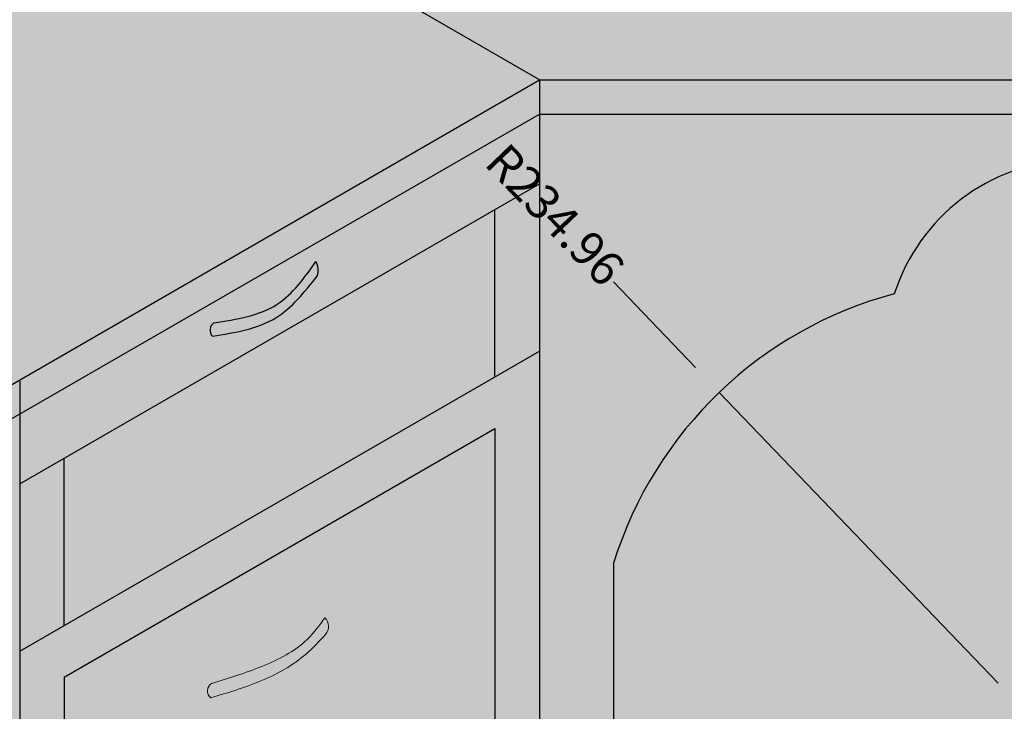
# Model space of a CAD drawing. Units: millimetres. Extents: x 78378 to 86415, y 148682 to 152721.
# Tile 8 of 18: x 79783 to 80358, y 150092 to 150495. Entities that reach past the tile are written whole.
import ezdxf

# ---------------------------------------------------------------- set-up
doc = ezdxf.new("R2010")
doc.units = ezdxf.units.MM
for name, color, linetype, lineweight in [('A-ANNO-DIMS', 2, 'Continuous', 18), ('A-FURN', 4, 'Continuous', 25), ('A-FURN-HRDW', 8, 'Continuous', 18), ('A-FURN-PATT', 32, 'Continuous', 13)]:
    doc.layers.add(name, color=color, linetype=linetype, lineweight=lineweight)
doc.styles.get("Standard").update_dxf_attribs({"font": 'arial.ttf'})
doc.dimstyles.new('ISO-25', dxfattribs={"dimtxt": 20, "dimasz": 20, "dimexe": 1.25, "dimexo": 0.625, "dimtad": 0, "dimdec": 1, "dimtxsty": 'Standard', "dimcen": 2.5, "dimadec": 0, "dimazin": 0, "dimtfac": 1, "dimtdec": 1, "dimtmove": 0, "dimatfit": 3, "dimfxl": 1, "dimarcsym": 0})

# ---------------------------------------------------------------- blocks, each defined once
blk = doc.blocks.new('HANDLE-DRAWER')
for centre, radius, start, end in [((63.38622997708444, 41.62154367045149), 7.231969022595942, 319.3237562697811, 44.69265733271547), ((5.163435732683865, 4.025219173752702), 5.172557027146686, 122.0794663418697, 231.0916038547452)]:
    blk.add_arc(centre, radius, start, end)
for points, knots in [([(2.416316796850878, 8.407990414794767), (12.22361058796001, 11.4080339887645), (31.81170594566225, 17.4000171857454), (55.97206586949582, 29.46692429189343), (65.30177131113433, 42.2784439569471), (68.52736162004294, 46.70781355843064)], [0, 0, 0, 0, 30.92804236988506, 61.77253950703249, 78.07166049105084, 78.07166049105084, 78.07166049105084, 78.07166049105084]), ([(1.914671141596045, 0.0001881390053313), (11.78696018195832, 2.942018891461464), (31.50487046795086, 8.817733694416148), (54.70585002572761, 21.54120260495396), (65.2835446695137, 33.01612223177024), (68.87098889380286, 36.90786192796077)], [0, 0, 0, 0, 30.92804236988506, 61.77253950704738, 77.60214595393334, 77.60214595393334, 77.60214595393334, 77.60214595393334])]:
    blk.add_open_spline(points, degree=3, knots=knots)
blk = doc.blocks.new('*D32')
at = {"layer": 'A-ANNO-DIMS', "color": 0, "lineweight": -2, "transparency": 16777216}
for p, q in [((80086.404202, 150459.382643), (80086.404202, 148693.757643)), ((80692.621985, 150459.382643), (80692.621985, 148693.757643)), ((80106.404202, 148695.007643), (80355.19095843862, 148695.007643)), ((80672.621985, 148695.007643), (80423.8352285614, 148695.007643))]:
    blk.add_line(p, q, dxfattribs=at)
at = {"layer": 'A-ANNO-DIMS', "color": 0, "transparency": 16777216}
for points in [[(80106.404202, 148698.3409763333), (80106.404202, 148691.6743096666), (80086.404202, 148695.007643)], [(80672.621985, 148698.3409763333), (80672.621985, 148691.6743096666), (80692.621985, 148695.007643)]]:
    blk.add_solid(points, dxfattribs=at)
at = {"layer": 'Defpoints', "color": 0, "transparency": 16777216}
for p in [(80086.404202, 150460.007643), (80692.621985, 150460.007643), (80692.621985, 148695.007643)]:
    blk.add_point(p, dxfattribs=at)
at = {"layer": 'A-ANNO-DIMS', "color": 0, "transparency": 16777216, "insert": (80389.5130935, 148695.007643), "char_height": 20, "attachment_point": 5}
blk.add_mtext('606.2', dxfattribs=at)
blk = doc.blocks.new('*D63')
at = {"layer": 'A-ANNO-DIMS', "color": 0, "lineweight": -2, "transparency": 16777216}
for p, q in [((80129.57071185744, 150342.1032015505), (80177.51998013844, 150292.103098691)), ((80353.993525, 150108.081617), (80191.36297800002, 150277.668023))]:
    blk.add_line(p, q, dxfattribs=at)
at = {"layer": 'A-ANNO-DIMS', "color": 0, "transparency": 16777216}
blk.add_solid([(80179.92582608695, 150294.4102650013), (80175.11413418995, 150289.7959323807), (80191.36297800002, 150277.668023)], dxfattribs=at)
at = {"layer": 'Defpoints', "color": 0, "transparency": 16777216}
for p in [(80191.36297800002, 150277.668023), (80353.993525, 150108.081617)]:
    blk.add_point(p, dxfattribs=at)
at = {"layer": 'A-ANNO-DIMS', "color": 0, "transparency": 16777216, "insert": (80093.78465023855, 150379.4198661427), "char_height": 20, "attachment_point": 5, "rotation": 313.8005333959761}
blk.add_mtext('R234.96', dxfattribs=at)

msp = doc.modelspace()

# ---------------------------------------------------------------- hatches: boundary and pattern name
at = {"layer": 'A-FURN-PATT'}
h = msp.add_hatch(color=256, dxfattribs=at)
h.dxf.hatch_style = 1
h.paths.add_polyline_path([(78839.32762104142, 151040.0076434961), (78579.5199999061, 151190.0076434961), (78579.51999990609, 150470.0076434961), (78839.3276210414, 150320.0076434962)])
h.paths.add_polyline_path([(79073.15448006323, 150899.6468812434, 0.2777796948118413), (79002.26445210895, 150996.320534414, 0.7910839311940991), (78917.95668085644, 150978.871860828, 0.1804483162531181), (78856.64812911711, 150853.0137915998), (78856.6481291171, 150350.6972986685), (79073.15448006321, 150484.3179883237)])
h.paths.add_polyline_path([(79073.15448006324, 151175.0076434962), (78856.64812911711, 151050.0076434961), (78856.64812911711, 150853.0137915998, -0.1804483162531142), (78917.95668085644, 150978.871860828, -0.7910839311941295), (79002.26445210895, 150996.320534414, -0.2777796948118357), (79073.15448006323, 150899.6468812434)])
h.paths.add_polyline_path([(79341.6223552364, 151350.0076434962), (79099.13524217675, 151490.0076434961), (78596.84050798177, 151200.0076434961), (78839.32762104142, 151060.0076434961)])
h.paths.add_polyline_path([(79904.53886769625, 151675.0076434962), (79662.05175463663, 151815.0076434961), (79099.13524217677, 151490.0076434961), (79341.62235523641, 151350.0076434962)])
h.paths.add_polyline_path([(80389.51309381555, 151955.0076434962), (80389.51309381555, 152235.0076434961), (79662.05175463663, 151815.0076434961), (79904.53886769625, 151675.0076434962)])
h.paths.add_polyline_path([(80389.51309381556, 151955.0076434962), (80164.3464888316, 151825.0076434962), (80164.3464888316, 151105.0076434962), (80614.67969879952, 151105.0076434962), (80614.6796987995, 151825.0076434962)])
edge = h.paths.add_edge_path(flags=16)
edge.add_spline(control_points=[(80216.30801305865, 151728.2510436129), (80227.18536059232, 151732.9809964381), (80256.33007611947, 151745.6544105326), (80298.40995723462, 151761.9595198717), (80340.25974320961, 151805.8549546823), (80391.07708467716, 151782.0404209196), (80454.03959007034, 151805.7580622626), (80496.50068603146, 151742.4094823368), (80543.82179764508, 151733.4042954735), (80562.71817457242, 151729.808323201)], knot_values=[0, 0, 0, 0, 35.54374676083332, 95.23575346876503, 136.367675126486, 200.9329819670103, 236.7264108107793, 322.8899349763893, 380.1702736670829, 380.1702736670829, 380.1702736670829, 380.1702736670829], degree=3, periodic=0)
edge.add_line((80562.71817457242, 151729.808323201), (80562.71817457245, 151165.0076434962))
edge.add_line((80562.71817457245, 151165.0076434962), (80216.30801305866, 151165.0076434962))
edge.add_line((80216.30801305866, 151165.0076434962), (80216.30801305865, 151728.2510436129))
h.paths.add_polyline_path([(80632.00020687516, 152095.0076434962), (80389.51309381555, 152235.0076434961), (80389.51309381555, 151955.0076434962), (80614.6796987995, 151825.0076434962), (80632.0002068752, 151815.0076434962)])
h.paths.add_polyline_path([(80867.77935513339, 151958.88048878), (80632.00020687516, 152095.0076434962), (80632.0002068752, 151815.0076434962), (80632.0002068752, 151510.0076434961), (80867.77935513335, 151373.88048878)])
h.paths.add_polyline_path([(80147.02598075592, 151495.8202891389, 0.1891897896548484), (80063.56711348135, 151597.7244306894, 0.7882613551016187), (79979.26906997921, 151580.5832085911, 0.1607261321771384), (79904.53886769625, 151413.5769349066), (79904.53886769625, 150955.0076434962), (80147.0259807559, 151095.0076434962)])
h.paths.add_polyline_path([(80147.02598075592, 151815.0076434961), (79904.53886769625, 151675.0076434962), (79904.53886769625, 151413.5769349066, -0.1607261321771371), (79979.26906997921, 151580.5832085911, -0.7882613551017736), (80063.56711348135, 151597.7244306894, -0.189189789654803), (80147.02598075592, 151495.820289139)])
h.paths.add_polyline_path([(79887.21835962054, 151645.0076434962), (79640.40111954202, 151502.5076434962), (79640.40111954202, 151262.3324568555, -0.160726132177166), (79715.13132182499, 151429.33873054, -0.7882613551016538), (79799.42936532712, 151446.4799526383, -0.2129057797217132), (79887.21835962054, 151328.7246881029)])
h.paths.add_polyline_path([(79799.42936532712, 151446.4799526383, 0.7882613551016341), (79715.13132182499, 151429.33873054, 0.1607261321772164), (79640.40111954202, 151262.3324568554), (79640.401119542, 150822.5076434962), (79887.21835962054, 150965.0076434962), (79887.21835962054, 151328.7246881029, 0.2129057797217146)])
h.paths.add_polyline_path([(79605.76010339064, 151482.5076434962), (79358.94286331208, 151340.0076434962), (79358.94286331208, 151100.0700856759, -0.1607261321769527), (79433.67306559504, 151267.0763593602, -0.7882613551016573), (79517.97110909715, 151284.2175814584, -0.2129057797218584), (79605.76010339064, 151166.4623169229)])
h.paths.add_polyline_path([(79605.76010339064, 151166.4623169229, 0.2129057797218619), (79517.97110909715, 151284.2175814584, 0.7882613551016192), (79433.67306559504, 151267.0763593602, 0.160726132177026), (79358.94286331208, 151100.0700856758), (79358.9428633121, 150742.9831021798), (79419.08774136574, 150694.7323050308), (79605.76010339062, 150802.5076434962)])
edge = h.paths.add_edge_path(flags=0)
edge.add_spline(control_points=[(81152.43559504113, 151098.7675637242), (81105.72083218757, 151145.9466131586), (81038.6136018851, 151213.7208057789), (80882.38658818699, 151214.1937625951), (80797.44342369089, 151311.2996726886), (80711.86856819791, 151340.3754369685), (80681.7690729932, 151350.6023409169)], knot_values=[0, 0, 0, 0, 188.2334409997391, 270.4032751997918, 445.4517920122014, 540.4285882874335, 540.4285882874335, 540.4285882874335, 540.4285882874335], degree=3, periodic=0)
edge.add_line((80683.45384528628, 151350.0268865391), (80683.45384528628, 151104.8791667058))
edge.add_line((80683.45384528628, 151104.8791667058), (81152.43559504113, 150851.3990036113))
edge.add_line((81152.43559504113, 150851.3990036113), (81152.43559504113, 151098.7675637242))
edge = h.paths.add_edge_path(flags=0)
edge.add_spline(control_points=[(80912.90176973268, 151027.1103287246), (80892.37419951524, 151034.1027281281), (80860.16629805118, 151045.073851773), (80835.5096829066, 151068.1214310134), (80826.56785747813, 151076.4797327879)], knot_values=[0, 0, 0, 0, 63.98405104007646, 100.3914242817051, 100.3914242817051, 100.3914242817051, 100.3914242817051], degree=3, periodic=0)
edge.add_arc((80830.04136161639, 151081.2991864332), 5.940737701461331, 100.92772760250938, 234.2187380998064, ccw=False)
edge.add_spline(control_points=[(80828.91517224, 151087.1322012562), (80837.85699766847, 151078.7738994817), (80862.513612813, 151055.7263202413), (80894.72151427707, 151044.7551965964), (80915.24908449454, 151037.7627971929)], knot_values=[0, 0, 0, 0, 36.40737324162872, 100.3914242817051, 100.3914242817051, 100.3914242817051, 100.3914242817051], degree=3, periodic=0)
edge.add_arc((80914.78821288893, 151032.2794977135), 5.50263353472094, -107.95403991859422, 85.19557899478139, ccw=False)
h.paths.add_polyline_path([(81238.21798952432, 151110.0076434962), (80632.0002068752, 151460.0076434962), (80632.00020687521, 151105.0076434962), (81238.21798952432, 150755.0076434961)])
edge = h.paths.add_edge_path(flags=16)
edge.add_line((81152.43559504113, 150851.3990036113), (80683.45384528628, 151104.8791667058))
edge.add_line((80683.45384528628, 151104.8791667058), (80683.45384528628, 151350.0278851498))
edge.add_spline(control_points=[(80681.7690729932, 151350.6023409169), (80711.86856819793, 151340.3754369685), (80797.44342369087, 151311.2996726885), (80882.38658818699, 151214.1937625951), (81038.61360188508, 151213.7208057789), (81105.72083218754, 151145.9466131586), (81152.43559504113, 151098.7675637242)], knot_values=[0, 0, 0, 0, 94.97679627523202, 270.0253130876416, 352.1951472876943, 540.4285882874335, 540.4285882874335, 540.4285882874335, 540.4285882874335], degree=3, periodic=0)
edge.add_line((81152.43559504113, 151098.7675637242), (81152.43559504113, 150851.3990036113))
edge = h.paths.add_edge_path(flags=0)
edge.add_spline(control_points=[(80912.90176973268, 151027.1103287246), (80892.37419951524, 151034.1027281281), (80860.16629805118, 151045.073851773), (80835.5096829066, 151068.1214310134), (80826.56785747813, 151076.4797327879)], knot_values=[0, 0, 0, 0, 63.98405104007646, 100.3914242817051, 100.3914242817051, 100.3914242817051, 100.3914242817051], degree=3, periodic=0)
edge.add_arc((80830.04136161639, 151081.2991864332), 5.940737701461331, 100.92772760250938, 234.2187380998064, ccw=False)
edge.add_spline(control_points=[(80828.91517224, 151087.1322012562), (80837.85699766847, 151078.7738994817), (80862.513612813, 151055.7263202413), (80894.72151427707, 151044.7551965964), (80915.24908449454, 151037.7627971929)], knot_values=[0, 0, 0, 0, 36.40737324162872, 100.3914242817051, 100.3914242817051, 100.3914242817051, 100.3914242817051], degree=3, periodic=0)
edge.add_arc((80914.78821288893, 151032.2794977135), 5.50263353472094, -107.74178823087311, 85.19557899478139, ccw=False)
h.paths.add_polyline_path([(81498.02561065964, 151255.0076434964), (81238.21798952432, 151110.0076434962), (81238.21798952432, 150755.0076434961), (81498.02561065964, 150905.0076434961)])
edge = h.paths.add_edge_path(flags=16)
edge.add_spline(control_points=[(81152.43559504113, 151098.7675637242), (81105.72083218757, 151145.9466131586), (81038.6136018851, 151213.7208057789), (80882.38658818699, 151214.1937625951), (80797.44342369089, 151311.2996726886), (80711.86856819791, 151340.3754369685), (80681.7690729932, 151350.6023409169)], knot_values=[0, 0, 0, 0, 188.2334409997391, 270.4032751997918, 445.4517920122014, 540.4285882874335, 540.4285882874335, 540.4285882874335, 540.4285882874335], degree=3, periodic=0)
edge.add_line((80683.45384528628, 151350.0278851498), (80683.45384528628, 151104.8791667058))
edge.add_line((80683.45384528628, 151104.8791667058), (81152.43559504113, 150851.3990036113))
edge.add_line((81152.43559504113, 150851.3990036113), (81152.43559504113, 151098.7675637242))
h.paths.add_polyline_path([(81453.99042063669, 151280.4313723099), (80867.77935513337, 151618.8804887802), (80867.77935513335, 151373.88048878), (81238.21798952432, 151160.0076434962)])
edge = h.paths.add_edge_path(flags=16)
edge.add_line((81189.23035884998, 151297.6373231461), (81114.41656350951, 151300.215424286))
edge.add_arc((81412.09668133054, 151394.0166835757), 312.1091616570752, 179.756930250193, 197.4900342341806, ccw=False)
edge.add_ellipse((81154.0183349007, 151392.0436487034), major_axis=(-54.02641628705902, 3.630104487441717), ratio=0.22179693447735, start_angle=0, end_angle=0.351798526980474, ccw=False)
edge.add_ellipse((81154.0183349007, 151392.0436487034), major_axis=(-54.02641628705902, 3.630104487441717), ratio=0.22179693447735, start_angle=180, end_angle=359.9999999999994, ccw=False)
edge.add_spline(control_points=[(81196.1844279047, 151321.9475927373), (81224.98016894507, 151347.1455424091), (81266.88460841302, 151383.8143662904), (81222.03544587504, 151387.0303756764), (81208.00556851825, 151388.036419373)], knot_values=[0, 0, 0, 0, 75.09175173428014, 109.275804386584, 109.275804386584, 109.275804386584, 109.275804386584], degree=3, periodic=0)
edge.add_arc((80751.91118424264, 151435.614496195), 458.5692540520198, 342.489160211778, 345.646172005802, ccw=False)
edge = h.paths.add_edge_path(flags=0)
edge.add_spline(control_points=[(81196.61933933741, 151323.6570128237), (81197.89298947518, 151324.7716730423), (81199.16543060394, 151325.8857721112), (81209.0232630699, 151334.5342782859), (81217.3958880952, 151341.9835067706), (81228.09276343176, 151352.5011683344), (81231.38832729329, 151355.9523700551), (81236.9492742566, 151362.4394637984), (81239.21399888789, 151365.4773121109), (81241.49874594079, 151369.4160429918), (81242.06403714154, 151370.554153099), (81242.91869346309, 151372.6971027681), (81243.20761616631, 151373.7015371057), (81243.50116908352, 151375.5538574188), (81243.50645821408, 151376.4000030934), (81243.24316774576, 151377.9407252098), (81242.97751237078, 151378.6372898393), (81242.14015699248, 151379.9370354702), (81241.5658612394, 151380.5415506406), (81240.20389796112, 151381.5329566703), (81239.49629055885, 151381.9384109359), (81237.06189936084, 151383.0663204191), (81235.02423457924, 151383.6998500153), (81230.35196602745, 151384.7569136921), (81227.71727859117, 151385.1826462377), (81221.91180586112, 151385.9145017437), (81218.71933734383, 151386.213257908), (81213.79120700595, 151386.611489939), (81212.12519739784, 151386.7359484812), (81209.61962229511, 151386.9181059123), (81208.78653612663, 151386.9778506286), (81207.90086381555, 151387.0431786834)], knot_values=[0.0154874367935492, 0.0154874367935492, 0.0154874367935492, 0.0154874367935492, 3.337879569258078, 3.337879569258078, 25.85130624162371, 25.85130624162371, 37.52811307983364, 37.52811307983364, 49.20491991804358, 49.20491991804358, 54.285093800687, 54.285093800687, 59.36526768333043, 59.36526768333043, 64.44544156597385, 64.44544156597385, 69.52561544861727, 69.52561544861727, 74.6057893312607, 74.6057893312607, 78.49366784748545, 78.49366784748545, 86.25567095319849, 86.25567095319849, 94.01767405891154, 94.01767405891154, 102.2022655586974, 102.2022655586974, 106.2945613085904, 106.2945613085904, 108.3252217467433, 108.3252217467433, 108.3252217467433, 108.3252217467433], degree=3, periodic=0)
edge = h.paths.add_edge_path(flags=16)
edge.add_arc((81034.17317896045, 151350.4692849881), 42.58223422336468, 231.2679035139937, 306.15184603107093, ccw=False)
edge.add_line((81007.5303374241, 151317.2517344113), (81007.5303374241, 151395.1810388082))
edge.add_ellipse((81033.41196842556, 151394.7791071004), major_axis=(-25.88163100145178, 0.4537615328445103), ratio=0.2389450898152861, start_angle=0, end_angle=0.1147075293308717, ccw=False)
edge.add_ellipse((81033.41196842556, 151394.7791071004), major_axis=(-25.88163100145178, 0.4537615328445103), ratio=0.2389450898152861, start_angle=181.1677708707583, end_angle=358.9476457193874, ccw=False)
edge.add_ellipse((81033.41196842556, 151395.7791071004), major_axis=(-25.88163100145178, 0.4537615328445103), ratio=0.2389450898152861, start_angle=179.9999999981626, end_angle=360.1147075293309, ccw=False)
edge.add_ellipse((81033.41196842556, 151395.7791071004), major_axis=(-25.88163100145178, 0.4537615328445103), ratio=0.2389450898152861, start_angle=178.9476457196991, end_angle=179.9999999981626, ccw=False)
edge.add_line((81059.293599427, 151395.1778229301), (81059.293599427, 151394.3771753934))
edge.add_ellipse((81033.41196842556, 151394.7791071004), major_axis=(-25.88163100145178, 0.4537615328445103), ratio=0.2389450898152861, start_angle=179.9999999981626, end_angle=180.1147075311684, ccw=False)
edge.add_ellipse((81033.41196842556, 151394.7791071004), major_axis=(-25.88163100145178, 0.4537615328445103), ratio=0.2389450898152861, start_angle=3.6903097823663984, end_angle=176.440650305715, ccw=False)
edge.add_line((81059.293599427, 151393.3387785743), (81059.293599427, 151316.0859874871))
h.paths.add_polyline_path([(80951.93545857484, 151343.9567836094), (80909.6837602833, 151362.463470517), (80904.02186617583, 151443.961481619, -0.3813330760227573), (80987.21689667807, 151411.3716886216)], flags=16)
h = msp.add_hatch(color=256, dxfattribs=at)
h.dxf.hatch_style = 1
h.paths.add_polyline_path([(80389.81355980314, 150935.1811176149), (80389.51309381555, 151105.0076434962), (80164.3464888316, 151105.0076434962), (79904.53886769625, 150955.0076434962), (79433.58476952511, 150683.1021681411), (79459.41281351625, 150662.3818050495), (79243.9048024148, 150537.9581968276), (79160.4069246431, 150518.167363956), (78839.3276210414, 150320.0076434962), (78579.51999990609, 150470.0076434961), (78570.85974586825, 150475.0076434961), (78570.85974586825, 150465.0076434962), (78570.85974586825, 149885.0076434961)])
h.paths.add_polyline_path([(80086.40420249099, 150460.0076434961), (79826.59658135568, 150610.0076434961), (78570.85974586825, 149885.0076434961), (78830.66736700358, 149735.0076434961)])
h.paths.add_polyline_path([(79540.80006404899, 150161.0556565937), (79217.39666007676, 149974.3386142535), (78980.9165707482, 150110.8704574853), (79304.31997472048, 150297.5874998256)], flags=16)
h.paths.add_polyline_path([(79506.15904789761, 150161.0556565937), (79217.39666007677, 149994.3386142535), (79015.55758689957, 150110.8704574853), (79304.31997472048, 150277.5874998256)], flags=0)
edge = h.paths.add_edge_path(flags=0)
edge.add_arc((79247.8635885932, 150177.154059363), 137.979927152229, 256.0025927560106, 293.5594108656914)
edge.add_arc((79240.76712928673, 150078.260535577), 68.08549769177299, 336.0991039681863, 387.369687653981)
edge.add_ellipse((79258.3073696606, 150109.4851683714), major_axis=(-42.62344506003415, -1.659142297571932), ratio=0.1604284291443649, start_angle=0, end_angle=179.0977278657225, ccw=False)
edge.add_arc((79285.21118690472, 150074.2509041072), 77.20964330046426, 155.1233103751286, 203.6557939001038)
edge = h.paths.add_edge_path(flags=0)
edge.add_ellipse((79258.69578401413, 150110.8297486024), major_axis=(-42.62344506003415, -1.659142297571932), ratio=0.1604284291443649, start_angle=350.6039411592706, end_angle=356.2289762200799)
edge.add_line((79219.16897707367, 150111.8937051806), (79218.32684768032, 150109.4140931549))
edge.add_arc((79262.46751974897, 150032.9602064517), 88.28134413732826, 112.39312291994881, 119.99999999999571, ccw=False)
h.paths.add_polyline_path([(79287.06250338514, 150086.9702731333, -0.247702064009433), (79288.19674658246, 150077.2955427019, -0.3904765126137986), (79265.47309673205, 150072.5437639662, -0.4872615262363024), (79264.07897218876, 150082.3768585209, 0.3956043262328261)], flags=0)
h.paths.add_polyline_path([(80389.51309381556, 150935.0076434961), (79826.59658135568, 150610.0076434961), (80086.40420249099, 150460.0076434961), (80692.6219851401, 150460.0076434961), (80952.42960627541, 150610.0076434961)])
edge = h.paths.add_edge_path(flags=16)
edge.add_ellipse((80392.44658491029, 150825.6009587087), major_axis=(-133.0756756189512, 7.721978101297283), ratio=0.424499569836956, start_angle=0, end_angle=360)
edge = h.paths.add_edge_path(flags=0)
edge.add_spline(control_points=[(80269.35411604258, 150832.7436415815), (80269.29193278665, 150831.6720147667), (80269.35031475963, 150830.592249842), (80269.73411879689, 150828.3360718096), (80270.06118209881, 150827.1586823489), (80271.04613754865, 150824.6748448987), (80271.70517726007, 150823.3691586005), (80273.40612032128, 150820.6503360826), (80274.44810410585, 150819.2381263036), (80276.93657810257, 150816.3508564802), (80278.3827638828, 150814.8762414973), (80282.58575216534, 150811.0913237019), (80285.62609899955, 150808.7701423959), (80292.60313446997, 150804.2267034199), (80296.53882829295, 150802.0041234762), (80305.19495220963, 150797.7581273222), (80309.91505114386, 150795.7343743789), (80320.0111596611, 150791.9599857595), (80325.38703862559, 150790.2091628441), (80339.21624322617, 150786.3149836253), (80347.95776464436, 150784.3563224224), (80366.06785395242, 150781.2568288573), (80375.43585590576, 150780.1158444778), (80394.309330179, 150778.7158311894), (80403.81420373028, 150778.4568170495), (80422.465596717, 150778.8319300563), (80431.61154730739, 150779.4662025667), (80449.06079653747, 150781.5837654722), (80457.36359407243, 150783.0675039467), (80472.6698529301, 150786.7766095128), (80479.67258750588, 150789.0032721294), (80490.18936031369, 150793.2813222805), (80494.12675567923, 150795.1967122277), (80501.0145611878, 150799.188512515), (80503.9631522054, 150801.2651387212), (80508.20659370373, 150804.9015163823), (80509.7300059309, 150806.4609393726), (80512.19955536906, 150809.4942049083), (80513.14558327098, 150810.9657349426), (80514.42909982229, 150813.5430698013), (80514.84355071915, 150814.6688389962), (80515.39838138374, 150816.8624682529), (80515.5404646545, 150817.9315158847), (80515.58008082317, 150820.0980035506), (80515.47732053277, 150821.197772811), (80514.99049560675, 150823.5061778107), (80514.6046629432, 150824.7154201442), (80513.48543938114, 150827.2641302181), (80512.7510921682, 150828.6026612985), (80510.88722780815, 150831.3808578872), (80509.75776214547, 150832.8196480674), (80507.0873051963, 150835.7513330261), (80505.5466409065, 150837.243857375), (80501.06238832264, 150841.0944478958), (80497.8199298022, 150843.4575549534), (80490.4173793454, 150848.0619874995), (80486.25822277585, 150850.3037143823), (80477.14480578042, 150854.5642972019), (80472.19085006021, 150856.583496544), (80461.6274878137, 150860.3244857693), (80456.01820904585, 150862.0464562905), (80441.73317330678, 150865.8126742317), (80432.78853232553, 150867.6675482482), (80414.33909310326, 150870.5316780972), (80404.8348928345, 150871.5410542788), (80385.7706775062, 150872.6572210053), (80376.21128671143, 150872.7639759942), (80357.54439280283, 150872.0728395342), (80348.43747055416, 150871.27476178), (80331.16822413795, 150868.8299635098), (80323.00642023917, 150867.1826714935), (80309.47200145545, 150863.5363064667), (80303.8627990537, 150861.6592748057), (80293.8018064812, 150857.5400855607), (80289.35122989668, 150855.2968623192), (80282.77569843757, 150851.2345481044), (80280.34726566746, 150849.4578867352), (80276.26060564672, 150845.9127204516), (80274.60404284154, 150844.1457946164), (80272.31573199967, 150841.1242619346), (80271.53575166185, 150839.8453762844), (80270.34961441216, 150837.3878672019), (80269.94168426798, 150836.2101260174), (80269.5065140611, 150834.2814629481), (80269.3988329965, 150833.5142652193), (80269.35411604258, 150832.7436415815)], knot_values=[0, 0, 0, 0, 0.0975004598125087, 0.0975004598125087, 0.1950009196250173, 0.1950009196250173, 0.2925013794375259, 0.2925013794375259, 0.3900018392500346, 0.3900018392500346, 0.4875022990625432, 0.4875022990625432, 0.6388032241337034, 0.6388032241337034, 0.7901041492048636, 0.7901041492048636, 0.9414050742760238, 0.9414050742760238, 1.092705999347184, 1.092705999347184, 1.312817101002443, 1.312817101002443, 1.532928202657702, 1.532928202657702, 1.753039304312961, 1.753039304312961, 1.973150405968221, 1.973150405968221, 2.19326150762348, 2.19326150762348, 2.413372609278739, 2.413372609278739, 2.569860632934037, 2.569860632934037, 2.726348656589336, 2.726348656589336, 2.844186581547077, 2.844186581547077, 2.962024506504818, 2.962024506504818, 3.060233875946405, 3.060233875946405, 3.158443245387991, 3.158443245387991, 3.256652614829578, 3.256652614829578, 3.354861984271164, 3.354861984271164, 3.453071353712751, 3.453071353712751, 3.551280723154337, 3.551280723154337, 3.649490092595923, 3.649490092595923, 3.803927730406353, 3.803927730406353, 3.958365368216782, 3.958365368216782, 4.112803006027212, 4.112803006027212, 4.267240643837642, 4.267240643837642, 4.489203494974081, 4.489203494974081, 4.711166346110521, 4.711166346110521, 4.93312919724696, 4.93312919724696, 5.155092048383399, 5.155092048383399, 5.377054899519838, 5.377054899519838, 5.557853608626545, 5.557853608626545, 5.738652317733252, 5.738652317733252, 5.872395555677483, 5.872395555677483, 6.006138793621714, 6.006138793621714, 6.109604996023907, 6.109604996023907, 6.2130711984261, 6.2130711984261, 6.283185307179586, 6.283185307179586, 6.283185307179586, 6.283185307179586], degree=3, periodic=0)
edge = h.paths.add_edge_path(flags=0)
edge.add_ellipse((80392.446576265, 150825.6009639553), major_axis=(-101.8397670786795, 3.392257208815831), ratio=0.403492477068114, start_angle=0, end_angle=360)
edge = h.paths.add_edge_path(flags=0)
edge.add_ellipse((80391.1657165424, 150858.3745518381), major_axis=(9.088237780547283, -0.67334552975693), ratio=0.3513541290445306, start_angle=0, end_angle=360)
h.paths.add_polyline_path([(80952.42960627541, 150610.0076434961), (80692.62198514014, 150460.0076434962), (81361.23421645904, 150073.9841917607), (81649.96279182703, 150052.7286159431), (81766.49348583283, 150120.0076434961), (81766.49348583283, 150140.0076434961), (81564.90245463562, 150256.396279624), (81564.88840704803, 150096.1962601479), (81538.90760017018, 150111.1962859926), (81538.92165266915, 150271.3963026331)])
h.paths.add_polyline_path([(81539.035680894, 151571.3304684069), (80867.77935513339, 151958.88048878), (80867.77935513337, 151618.8804887802), (81498.02561065964, 151255.0076434964), (81498.02561065964, 150905.0076434961), (81238.21798952435, 150755.0076434961), (81538.94884401507, 150581.3806037023)])
h.paths.add_polyline_path([(81766.49348583283, 151440.0076434962), (81565.01644300755, 151556.3304684069), (81564.92963647815, 150566.38058618), (81766.49348583283, 150450.0076434962)])
edge = h.paths.add_edge_path()
edge.add_line((81564.92963647815, 150566.38058618), (81564.9136990684, 150384.628856009))
edge.add_ellipse((81552.13037602534, 150358.5718270642), major_axis=(52.62721254190076, 3.506026927036754), ratio=0.4958990548584225, start_angle=367.51697565131457, end_angle=420.0564685523974, ccw=False)
edge.add_ellipse((81552.13037602534, 150358.5718270642), major_axis=(52.62721254190076, 3.506026927036754), ratio=0.4958990548584225, start_angle=351.72974196033346, end_angle=367.51697565131457, ccw=False)
edge.add_ellipse((81552.13037602534, 150345.5015529042), major_axis=(52.62721254190076, 3.506026927036754), ratio=0.4958990548584225, start_angle=352.51169489415116, end_angle=366.30060915387577, ccw=False)
edge.add_line((81603.4463374456, 150342.2038825707), (81603.50642755294, 150340.4474978293))
edge.add_ellipse((81552.13037602534, 150332.1280359686), major_axis=(52.62721254190076, 3.506026927036754), ratio=0.4958990548584225, start_angle=353.6729654395227, end_angle=365.38679972494066, ccw=False)
edge.add_ellipse((81552.13037602534, 150332.1280359686), major_axis=(52.62721254190076, 3.506026927036754), ratio=0.4958990548584225, start_angle=350.9388331002564, end_angle=353.6729654395227)
edge.add_line((81603.86882368504, 150329.8549549892), (81604.0441546891, 150324.7301729966))
edge.add_ellipse((81552.13037602534, 150317.7418284518), major_axis=(52.62721254190076, 3.506026927036754), ratio=0.4958990548584225, start_angle=355.21767463173103, end_angle=363.85533637812415, ccw=False)
edge.add_ellipse((81552.13037602534, 150317.7418284518), major_axis=(52.62721254190076, 3.506026927036754), ratio=0.4958990548584225, start_angle=341.3250873036158, end_angle=355.21767463173103, ccw=False)
edge.add_ellipse((81552.13037602534, 150317.7418284518), major_axis=(52.62721254190076, 3.506026927036754), ratio=0.4958990548584225, start_angle=293.4661701367695, end_angle=341.3250873036158, ccw=False)
edge.add_line((81564.90566138821, 150292.9663898651), (81564.90245463562, 150256.396279624))
edge.add_line((81564.90245463562, 150256.396279624), (81766.49348583283, 150140.0076434961))
edge.add_line((81766.49348583283, 150140.0076434961), (81766.49348583283, 150450.0076434962))
edge.add_line((81766.49348583283, 150450.0076434962), (81564.92963647815, 150566.38058618))
h.paths.add_polyline_path([(81525.57129610774, 150321.5980043728), (81526.59848255829, 150321.3069082928), (81528.6771290606, 150320.947049251)])
h.paths.add_polyline_path([(81512.79027333307, 150326.1128631878), (81514.50580755486, 150325.38873887), (81512.53799543541, 150326.2678422534)])
h.paths.add_polyline_path([(81533.21477271736, 150320.1614841748), (81534.69519629495, 150319.9051905676), (81536.59953044976, 150319.755668921)])
h.paths.add_polyline_path([(81518.62200466282, 150323.6512984944), (81519.22704244989, 150323.3959129888), (81521.28902816366, 150322.8115634216)])
h.paths.add_polyline_path([(81501.21834684846, 150336.259909523), (81500.35429342867, 150338.133928838), (81499.78149159584, 150340.0493926212), (81499.50316348342, 150341.9955259773), (81499.50316348343, 150343.7256661642), (81499.75838934928, 150345.5905095656), (81500.27655404429, 150347.4549063508), (81501.05505607055, 150349.3094961287), (81501.09670215519, 150349.3936770376), (81501.13888119749, 150349.4778172982), (81500.99777251929, 150349.749637304), (81500.86282558287, 150350.0225204294), (81499.50316348342, 150355.0658001372), (81499.95910976747, 150359.5002298216), (81501.89819062682, 150363.9082666975), (81505.26528150582, 150368.1645982632), (81509.96466211145, 150372.148224724), (81515.86273756725, 150375.7458987972), (81522.79183627458, 150378.8553451273), (81530.55497651099, 150381.3881677888), (81538.93146626501, 150383.2723632221), (81538.94884401507, 150581.3806037023), (80632.00020687521, 151105.0076434962), (80389.51309381555, 151105.0076434962), (80389.81417426979, 150934.8338146148), (80952.42960627541, 150610.0076434961), (81538.92165266915, 150271.3963026331), (81538.92343538092, 150291.719410528), (81538.87516273293, 150291.7210326448), (81530.1914951021, 150292.8238998863), (81522.18015347481, 150294.6903872688), (81515.08664870211, 150297.2632955209), (81509.86347084012, 150299.9959433281), (81505.6084410237, 150303.1350709547), (81502.41902318504, 150306.608774857), (81500.3682727948, 150310.3374878268), (81499.50316348343, 150314.2358015248), (81499.50316348343, 150315.9659417118), (81499.82059494797, 150318.1159244827), (81500.4869945128, 150320.2634115907), (81501.49791650465, 150322.3940767571), (81500.48699451279, 150324.4232810552), (81499.82059494796, 150326.50388518), (81499.50316348343, 150328.6220090417), (81499.50316348343, 150330.3521492286), (81499.78149159584, 150332.3262168982), (81500.35429342862, 150334.2991697576)])
h = msp.add_hatch(color=256, dxfattribs=at)
h.dxf.hatch_style = 1
h.paths.add_polyline_path([(79090.47498813891, 151205.0076434961), (78839.32762104142, 151060.0076434961), (78839.3276210414, 150320.0076434962), (79090.4749881389, 150475.0076434961)])
h.paths.add_polyline_path([(79073.15448006324, 151175.0076434962), (79073.15448006323, 150899.6468812434, -0.0454436300045199), (79073.15448006323, 150878.5652698783), (79073.15448006321, 150484.3179883237), (78856.6481291171, 150350.6972986685), (78856.64812911711, 150814.5249476813, -0.0481571609008244), (78856.64812911711, 150853.0137915998), (78856.64812911711, 151050.0076434961)], flags=16)
h.paths.add_polyline_path([(79358.94286331208, 151340.0076434962), (79605.76010339064, 151482.5076434962), (79605.76010339062, 150802.5076434962), (79419.08774136574, 150694.7323050308), (79433.58476952511, 150683.1021681411), (79623.08061146631, 150792.5076434962), (79623.08061146631, 151512.5076434962), (79341.6223552364, 151350.0076434962), (79341.6223552364, 150756.8783555866), (79358.9428633121, 150742.9831021798)])
h.paths.add_polyline_path([(79341.6223552364, 151350.0076434962), (79090.47498813891, 151205.0076434961), (79090.4749881389, 150475.0076434961), (79160.4069246431, 150518.167363956), (79107.79549621459, 150505.6972986686), (79107.79549621459, 151195.0076434962), (79109.52754702215, 151196.0076434962), (79324.3018471607, 151320.0076434962), (79324.30184716069, 150770.7736089934), (79341.6223552364, 150756.8783555866)])
h.paths.add_polyline_path([(79887.21835962054, 151645.0076434962), (79887.21835962054, 151665.0076434962), (79623.08061146631, 151512.5076434962), (79623.08061146631, 150792.5076434962), (79887.21835962054, 150945.0076434962), (79887.21835962054, 150965.0076434962), (79640.401119542, 150822.5076434962), (79640.40111954202, 151502.5076434962)])
h.paths.add_polyline_path([(79904.53886769625, 151655.0076434962), (79887.21835962054, 151645.0076434962), (79887.21835962054, 150965.0076434962), (79904.53886769625, 150975.0076434962)])
h.paths.add_polyline_path([(80164.3464888316, 151825.0076434962), (80147.02598075592, 151815.0076434961), (80147.0259807559, 151095.0076434962), (80164.3464888316, 151105.0076434962)])
h.paths.add_polyline_path([(80632.0002068752, 151510.0076434961), (80632.0002068752, 151490.0076434962), (81238.21798952432, 151140.0076434962), (81471.60449664589, 151270.2618807845), (81453.99042063669, 151280.4313723099), (81238.21798952432, 151160.0076434962)])
h.paths.add_polyline_path([(80632.0002068752, 151490.0076434962), (80632.0002068752, 151470.0076434962), (81238.21798952432, 151120.0076434962), (81489.21857265507, 151260.092389259), (81471.60449664589, 151270.2618807845), (81238.21798952432, 151140.0076434962)])
h.paths.add_polyline_path([(80632.0002068752, 151460.0076434962), (80632.00020687521, 151105.0076434962), (81238.21798952432, 150755.0076434961), (81238.21798952432, 151110.0076434962)])
edge = h.paths.add_edge_path(flags=16)
edge.add_spline(control_points=[(80681.7690729932, 151350.6023409169), (80711.86856819793, 151340.3754369685), (80797.44342369087, 151311.2996726885), (80882.38658818699, 151214.1937625951), (81038.61360188508, 151213.7208057789), (81105.72083218754, 151145.9466131586), (81152.43559504113, 151098.7675637242)], knot_values=[0, 0, 0, 0, 94.97679627523202, 270.0253130876416, 352.1951472876943, 540.4285882874335, 540.4285882874335, 540.4285882874335, 540.4285882874335], degree=3, periodic=0)
edge.add_line((81152.43559504113, 151098.7675637242), (81152.43559504113, 150851.3990036113))
edge.add_line((81152.43559504113, 150851.3990036113), (80683.45384528628, 151104.8791667058))
edge.add_line((80683.45384528628, 151104.8791667058), (80683.45384528628, 151350.0270476502))
edge = h.paths.add_edge_path(flags=0)
edge.add_spline(control_points=[(80828.91517224, 151087.1322012562), (80837.85699766847, 151078.7738994817), (80862.513612813, 151055.7263202413), (80894.72151427707, 151044.7551965964), (80915.24908449454, 151037.7627971929)], knot_values=[0, 0, 0, 0, 36.40737324162872, 100.3914242817051, 100.3914242817051, 100.3914242817051, 100.3914242817051], degree=3, periodic=0)
edge.add_arc((80914.78821288893, 151032.2794977135), 5.50263353472094, -107.95403991859422, 85.19557899478139, ccw=False)
edge.add_spline(control_points=[(80912.90176973268, 151027.1103287246), (80892.37419951524, 151034.1027281281), (80860.16629805118, 151045.073851773), (80835.5096829066, 151068.1214310134), (80826.56785747813, 151076.4797327879)], knot_values=[0, 0, 0, 0, 63.98405104007646, 100.3914242817051, 100.3914242817051, 100.3914242817051, 100.3914242817051], degree=3, periodic=0)
edge.add_arc((80830.04136161639, 151081.2991864332), 5.940737701461332, 100.92772760250938, 234.2187380998064, ccw=False)
h.paths.add_polyline_path([(80632.0002068752, 151815.0076434962), (80614.6796987995, 151825.0076434962), (80614.67969879952, 151105.0076434962), (80632.00020687521, 151105.0076434962)])
h.paths.add_polyline_path([(81498.02561065964, 151255.0076434964), (81489.21857265507, 151260.092389259), (81238.21798952432, 151120.0076434962), (80632.0002068752, 151470.0076434962), (80632.0002068752, 151460.0076434962), (81238.21798952432, 151110.0076434962)])
h.paths.add_polyline_path([(78596.84050798177, 151200.0076434961), (78579.51999990609, 151190.0076434961), (78839.32762104142, 151040.0076434961), (78839.32762104142, 151060.0076434961)])
h.paths.add_polyline_path([(78596.84050798177, 151200.0076434961), (78579.5199999061, 151210.0076434961), (78579.5199999061, 151190.0076434961)])
h.paths.add_polyline_path([(78579.5199999061, 151210.0076434961), (78570.85974586825, 151205.0076434961), (78570.85974586825, 150475.0076434961), (78579.51999990609, 150470.0076434961)])
h = msp.add_hatch(color=256, dxfattribs=at)
h.dxf.hatch_style = 1
h.paths.add_polyline_path([(79783.29531116647, 150265.0076434962), (79783.29531116647, 150285.0076434962), (79257.85559544402, 149981.6448821809), (79257.85559544402, 149961.6448821809)])
h.paths.add_polyline_path([(80086.40420249102, 150440.0076434961), (80086.40420249102, 150460.0076434962), (79783.29531116647, 150285.0076434962), (79783.29531116647, 150265.0076434962)])
h = msp.add_hatch(color=256, dxfattribs=at)
h.dxf.hatch_style = 1
h.paths.add_polyline_path([(80692.6219851401, 150460.0076434961), (80086.40420249102, 150460.0076434961), (80086.40420249102, 150440.0076434962), (80692.6219851401, 150440.0076434962)])
h = msp.add_hatch(color=256, dxfattribs=at)
h.dxf.hatch_style = 1
h.paths.add_polyline_path([(80692.6219851401, 150440.0076434962), (80086.40420249102, 150440.0076434962), (80086.40420249104, 149630.0076434962), (80692.62198514013, 149614.0076434961)])
h.paths.add_polyline_path([(80293.42096661613, 150335.1041026971, -0.693913746763918), (80505.02836664302, 150344.7159628166, -0.266337996674739), (80649.3207149509, 150178.1038520679), (80649.32071495091, 149665.150500639), (80129.70547268025, 149678.8647863533), (80129.70547268025, 150178.1038520678, -0.257326206066023)], flags=16)
h.paths.add_polyline_path([(80060.4234403775, 150384.3023755343), (79809.27607328002, 150239.3023755343), (79809.27607328001, 150141.6366131478), (80060.4234403775, 150286.6366131478)])
h.paths.add_polyline_path([(80086.40420249102, 150399.3023755343), (80086.40420249102, 150440.0076434961), (79783.29531116647, 150265.0076434962), (79783.29531116647, 150224.3023755343)])
edge = h.paths.add_edge_path(flags=16)
edge.add_arc((79946.63023943067, 150348.8762810125), 10.76362312575662, -18.381796908867102, 28.033199430885304, ccw=False)
edge.add_spline(control_points=[(79956.8446621052, 150345.4819987291), (79949.48615957417, 150336.2391268092), (79933.85278209679, 150316.6023454005), (79908.95072794275, 150312.561963116), (79895.76986639632, 150310.4233556278)], knot_values=[0, 0, 0, 0, 34.22568399180864, 72.71357657474474, 72.71357657474474, 72.71357657474474, 72.71357657474474], degree=3, periodic=0)
edge.add_arc((79899.38686741845, 150314.0155032977), 5.097668219542309, 123.6496152582665, 224.8024750763005, ccw=False)
edge.add_spline(control_points=[(79896.56218517898, 150318.2590149947), (79909.86104355381, 150320.2802713686), (79934.78207045459, 150324.0679487052), (79949.34122059586, 150344.4361083294), (79956.13102493295, 150353.9350019607)], knot_values=[0, 0, 0, 0, 38.48789258293611, 72.12331911350849, 72.12331911350849, 72.12331911350849, 72.12331911350849], degree=3, periodic=0)
h.paths.add_polyline_path([(80086.40420249102, 150399.3023755343), (80060.4234403775, 150384.3023755343), (80060.4234403775, 150286.6366131478), (80086.40420249102, 150301.6366131477)], flags=17)
h.paths.add_polyline_path([(79809.27607328002, 150239.3023755343), (79783.29531116647, 150224.3023755343), (79783.29531116647, 150126.6366131478), (79809.27607328001, 150141.6366131478)])
h = msp.add_hatch(color=256, dxfattribs=at)
h.dxf.hatch_style = 1
h.paths.add_polyline_path([(80060.4234403775, 150256.6366131478), (79809.27607328001, 150111.6366131478), (79809.27607328001, 149835.822128322), (80060.4234403775, 149980.822128322)])
edge = h.paths.add_edge_path(flags=16)
edge.add_arc((79897.98743573268, 150103.5556037615), 5.172557027142873, 122.07946634250479, 231.0916038546426, ccw=False)
edge.add_spline(control_points=[(79895.24031679684, 150107.9383750026), (79905.04761058795, 150110.9384185765), (79924.63570594566, 150116.9304017735), (79948.79606586948, 150128.9973088797), (79958.12577131113, 150141.8088285447), (79961.35136162004, 150146.2381981462)], knot_values=[0, 0, 0, 0, 30.92804236988506, 61.77253950703249, 78.07166049105084, 78.07166049105084, 78.07166049105084, 78.07166049105084], degree=3, periodic=0)
edge.add_arc((79956.21022997708, 150141.1519282582), 7.231969022599169, -40.6762437318896, 44.692657332507395, ccw=False)
edge.add_spline(control_points=[(79961.6949888938, 150136.4382465157), (79958.1075446695, 150132.5465068195), (79947.5298500257, 150121.0715871927), (79924.32887046793, 150108.3481182822), (79904.61096018193, 150102.4724034792), (79894.73867114159, 150099.5305727268)], knot_values=[0, 0, 0, 0, 15.82960644688596, 46.67410358404827, 77.60214595393333, 77.60214595393333, 77.60214595393333, 77.60214595393333], degree=3, periodic=0)
h.paths.add_polyline_path([(80060.4234403775, 149950.8221283219), (79809.27607328001, 149805.822128322), (79809.27607328001, 149500.0076434962), (80060.42344037753, 149645.0076434962)])
h.paths.add_polyline_path([(80649.3207149509, 150178.1038520679, 0.2663379966747387), (80505.02836664302, 150344.7159628166, 0.6939137467639167), (80293.42096661613, 150335.1041026971, 0.2573262060660234), (80129.70547268025, 150178.1038520678), (80129.70547268025, 149678.8647863533), (80649.32071495091, 149665.150500639)])
h = msp.add_hatch(color=256, dxfattribs=at)
h.dxf.hatch_style = 1
edge = h.paths.add_edge_path()
edge.add_spline(control_points=[(79895.76986639632, 150310.4233556278), (79908.95072794273, 150312.561963116), (79933.85278209682, 150316.6023454005), (79949.48615957418, 150336.2391268092), (79956.8446621052, 150345.4819987291)], knot_values=[0, 0, 0, 0, 38.48789258293611, 72.71357657474474, 72.71357657474474, 72.71357657474474, 72.71357657474474], degree=3, periodic=0)
edge.add_arc((79946.63023943067, 150348.8762810125), 10.76362312575662, 341.6182030911329, 388.0331994310585)
edge.add_spline(control_points=[(79956.13102493295, 150353.9350019607), (79949.34122059584, 150344.4361083293), (79934.78207045457, 150324.0679487052), (79909.86104355381, 150320.2802713686), (79896.56218517898, 150318.2590149947)], knot_values=[0, 0, 0, 0, 33.63542653057237, 72.12331911350849, 72.12331911350849, 72.12331911350849, 72.12331911350849], degree=3, periodic=0)
edge.add_arc((79899.38686741845, 150314.0155032977), 5.097668219542307, 123.6496152582664, 224.8024750763005)
h = msp.add_hatch(color=256, dxfattribs=at)
h.dxf.hatch_style = 1
h.paths.add_polyline_path([(79765.97480309076, 149445.0076434962), (79765.97480309078, 149603.6183766167), (79275.17610351968, 149320.2556153015), (79275.17610351968, 149161.6448821809), (79350.28260927423, 149205.0076434961)])
edge = h.paths.add_edge_path(flags=16)
edge.add_arc((79507.24398653943, 149406.7325176549), 51.45725872682493, 189.4892033869566, 208.9818028088169, ccw=False)
edge.add_spline(control_points=[(79456.49083369225, 149398.249183891), (79490.7805017203, 149406.8496318209), (79544.66821365236, 149420.3656116243), (79585.61673544894, 149461.098953088), (79597.20784070941, 149478.6256589295), (79597.88663588953, 149479.65205315)], knot_values=[0, 0, 0, 0, 103.8711517509291, 163.2380546532031, 166.9309452742424, 166.9309452742424, 166.9309452742424, 166.9309452742424], degree=3, periodic=0)
edge.add_arc((79598.46803720549, 149470.6288681557), 9.041896644556108, -55.21570256624602, 93.686708761847, ccw=False)
edge.add_spline(control_points=[(79603.62633526741, 149463.2027079073), (79602.94754008728, 149462.1763136868), (79591.3564348269, 149444.6496078453), (79550.40791303018, 149403.9162663817), (79496.52020109817, 149390.4002865783), (79462.23053307013, 149381.7998386483)], knot_values=[0, 0, 0, 0, 3.692890621039242, 63.05979352331328, 166.9309452742424, 166.9309452742424, 166.9309452742424, 166.9309452742424], degree=3, periodic=0)
h.paths.add_polyline_path([(80060.4234403775, 149980.822128322), (80060.4234403775, 150256.6366131478), (79809.27607328001, 150111.6366131478), (79809.27607328001, 149835.822128322)], flags=0)
edge = h.paths.add_edge_path(flags=0)
edge.add_arc((79897.98743573268, 150103.5556037615), 5.172557027142874, 122.07946634250479, 231.0916038545171, ccw=False)
edge.add_spline(control_points=[(79895.24031679684, 150107.9383750026), (79905.04761058795, 150110.9384185765), (79924.63570594566, 150116.9304017735), (79948.79606586948, 150128.9973088797), (79958.12577131113, 150141.8088285447), (79961.35136162004, 150146.2381981462)], knot_values=[0, 0, 0, 0, 30.92804236988506, 61.77253950703249, 78.07166049105084, 78.07166049105084, 78.07166049105084, 78.07166049105084], degree=3, periodic=0)
edge.add_arc((79956.21022997708, 150141.1519282582), 7.231969022599169, -40.6762437318896, 44.692657332507395, ccw=False)
edge.add_spline(control_points=[(79961.6949888938, 150136.4382465157), (79958.1075446695, 150132.5465068195), (79947.5298500257, 150121.0715871927), (79924.32887046793, 150108.3481182822), (79904.61096018193, 150102.4724034792), (79894.73867114159, 150099.5305727268)], knot_values=[0, 0, 0, 0, 15.82960644688596, 46.67410358404827, 77.60214595393333, 77.60214595393333, 77.60214595393333, 77.60214595393333], degree=3, periodic=0)
h.paths.add_polyline_path([(80060.4234403775, 149950.8221283219), (79809.27607328001, 149805.822128322), (79809.27607328001, 149500.0076434962), (80060.42344037753, 149645.0076434962)], flags=0)
edge = h.paths.add_edge_path(flags=0)
edge.add_arc((79897.98743573268, 149795.6302191737), 5.172557027142842, 122.07946634250479, 231.0916038545171, ccw=False)
edge.add_spline(control_points=[(79895.24031679684, 149800.0129904148), (79905.04761058795, 149803.0130339888), (79924.63570594566, 149809.0050171857), (79948.79606586948, 149821.0719242919), (79958.12577131113, 149833.883443957), (79961.35136162004, 149838.3128135584)], knot_values=[0, 0, 0, 0, 30.92804236988506, 61.77253950703249, 78.07166049105084, 78.07166049105084, 78.07166049105084, 78.07166049105084], degree=3, periodic=0)
edge.add_arc((79956.21022997708, 149833.2265436705), 7.231969022599074, -40.6762437318896, 44.692657332507395, ccw=False)
edge.add_spline(control_points=[(79961.6949888938, 149828.5128619279), (79958.1075446695, 149824.6211222318), (79947.5298500257, 149813.1462026049), (79924.32887046793, 149800.4227336944), (79904.61096018193, 149794.5470188914), (79894.73867114159, 149791.605188139)], knot_values=[0, 0, 0, 0, 15.82960644688596, 46.67410358404827, 77.60214595393333, 77.60214595393333, 77.60214595393333, 77.60214595393333], degree=3, periodic=0)
h.paths.add_polyline_path([(80086.40420249102, 150301.6366131477), (79783.29531116647, 150126.6366131478), (79783.29531116645, 149455.0076434962), (80086.40420249104, 149630.0076434962)])
h.paths.add_polyline_path([(79809.27607328001, 150111.6366131478), (80060.4234403775, 150256.6366131478), (80060.4234403775, 149980.822128322), (79809.27607328001, 149835.822128322)], flags=16)
h.paths.add_polyline_path([(80060.4234403775, 149950.8221283219), (80060.42344037753, 149645.0076434962), (79809.27607328001, 149500.0076434962), (79809.27607328001, 149805.822128322)], flags=16)
h = msp.add_hatch(color=256, dxfattribs=at)
h.dxf.hatch_style = 1
h.paths.add_polyline_path([(79765.97480309078, 150214.3023755343), (79275.17610351971, 149930.939614219), (79275.17610351968, 149340.2556153015), (79361.10187436163, 149389.8648822274), (79361.10187436163, 149854.0251874417), (79688.53915659874, 150043.071190484), (79688.53915659874, 149578.9108852697), (79765.97480309078, 149623.6183766168)], flags=0)
h.paths.add_polyline_path([(79616.99747211508, 150064.3357852431, -1), (79579.57778226466, 150064.3357852431, -1)], flags=0)
h.paths.add_polyline_path([(79511.25702160504, 150003.2865076769, -1), (79473.83733175462, 150003.2865076769, -1)], flags=0)
h.paths.add_polyline_path([(79398.61463104078, 149938.2523931624, -1), (79361.19494119036, 149938.2523931624, -1)], flags=0)
h.paths.add_polyline_path([(79688.53915659874, 149578.9108852697), (79667.16069404285, 149674.8368362752), (79401.25237372774, 149521.3145959615), (79361.10187436163, 149389.8648822274)], flags=0)
h.paths.add_polyline_path([(79783.29531116645, 149613.6183766167), (79783.29531116647, 150126.6366131478), (79783.29531116647, 150265.0076434962), (79257.85559544402, 149961.6448821809), (79257.85559544401, 149310.2556153015)])
h.paths.add_polyline_path([(79275.17610351968, 149340.2556153015), (79275.17610351971, 149930.939614219), (79765.97480309078, 150214.3023755343), (79765.97480309078, 149623.6183766168)], flags=16)
h.paths.add_polyline_path([(79361.10187436163, 149389.8648822274), (79361.10187436163, 149854.0251874417), (79688.53915659874, 150043.071190484), (79688.53915659874, 149578.9108852697), (79667.16069404285, 149674.8368362752), (79401.25237372774, 149521.3145959615)], flags=0)
h.paths.add_polyline_path([(79477.90289169294, 149864.6773096294), (79477.90289169294, 149877.6075739832), (79571.78517238796, 149931.8105340146), (79571.78517238796, 149918.8802696608)], flags=0)
h = msp.add_hatch(color=256, dxfattribs=at)
h.dxf.hatch_style = 1
edge = h.paths.add_edge_path()
edge.add_spline(control_points=[(79894.73867114159, 150099.5305727268), (79904.61096018193, 150102.4724034792), (79924.32887046794, 150108.3481182822), (79947.5298500257, 150121.0715871927), (79958.10754466952, 150132.5465068196), (79961.6949888938, 150136.4382465157)], knot_values=[0, 0, 0, 0, 30.92804236988506, 61.77253950704738, 77.60214595393334, 77.60214595393334, 77.60214595393334, 77.60214595393334], degree=3, periodic=0)
edge.add_arc((79956.21022997708, 150141.1519282582), 7.231969022599169, 319.3237562676103, 404.6926573325073)
edge.add_spline(control_points=[(79961.35136162004, 150146.2381981462), (79958.12577131113, 150141.8088285447), (79948.7960658695, 150128.9973088797), (79924.63570594563, 150116.9304017735), (79905.04761058795, 150110.9384185765), (79895.24031679684, 150107.9383750026)], knot_values=[0, 0, 0, 0, 16.29912098401835, 47.14361812116577, 78.07166049105084, 78.07166049105084, 78.07166049105084, 78.07166049105084], degree=3, periodic=0)
edge.add_arc((79897.98743573268, 150103.5556037615), 5.172557027142874, 122.0794663425048, 231.0916038545171)

# ---------------------------------------------------------------- linework, layer by layer
at = {"layer": 'A-FURN'}
for p, q in [((80086.40420249102, 150460.0076434961), (79826.59658135568, 150610.0076434961)), ((78830.66736700358, 149735.0076434961), (80086.40420249102, 150460.0076434962)), ((80086.40420249102, 150460.0076434962), (80086.40420249104, 149630.0076434962)), ((80086.40420249102, 150460.0076434961), (80692.6219851401, 150460.0076434961)), ((79257.85559544402, 149961.6448821809), (80086.40420249102, 150440.0076434961)), ((80086.40420249102, 150440.0076434962), (80692.6219851401, 150440.0076434962)), ((79783.29531116647, 150224.3023755343), (80086.40420249102, 150399.3023755343)), ((80060.4234403775, 150286.6366131478), (80060.4234403775, 150384.3023755343)), ((79783.29531116647, 150126.6366131478), (80086.40420249102, 150301.6366131477)), ((79783.29531116647, 150285.0076434961), (79783.29531116645, 149455.0076434961)), ((79809.27607328001, 150111.6366131478), (80060.4234403775, 150256.6366131478)), ((80060.4234403775, 150256.6366131478), (80060.4234403775, 149980.822128322)), ((79809.27607328001, 150141.6366131478), (79809.27607328002, 150239.3023755343)), ((80129.70547268025, 150178.1038520678), (80129.70547268025, 149678.8647863533)), ((79783.29531116647, 150126.6366131478), (79783.29531116645, 149455.0076434962)), ((79809.27607328001, 150111.6366131478), (79809.27607328001, 149835.822128322))]:
    msp.add_line(p, q, dxfattribs=at)
for centre, radius, start, end in [((80401.0201321819, 150300.382429083), 113.0627040584925, 23.08613834522145, 162.1153879537537), ((79946.63023943065, 150348.8762810125), 10.76362312577366, 341.6182030911573, 28.03319943092171), ((80353.9935247376, 150108.08161735), 234.9643454878818, 104.9392463657244, 162.6617514398103), ((79899.38686741845, 150314.0155032977), 5.09766821953428, 123.6496152582664, 224.8024750761852)]:
    msp.add_arc(centre, radius, start, end, dxfattribs=at)
for points, knots in [([(79896.56218517898, 150318.2590149947), (79909.86104355381, 150320.2802713686), (79934.78207045459, 150324.0679487052), (79949.34122059586, 150344.4361083294), (79956.13102493295, 150353.9350019607)], [0, 0, 0, 0, 38.48789258293611, 72.12331911350849, 72.12331911350849, 72.12331911350849, 72.12331911350849]), ([(79895.76986639632, 150310.4233556278), (79908.95072794273, 150312.561963116), (79933.85278209682, 150316.6023454005), (79949.48615957418, 150336.2391268092), (79956.8446621052, 150345.4819987291)], [0, 0, 0, 0, 38.48789258293611, 72.71357657474474, 72.71357657474474, 72.71357657474474, 72.71357657474474])]:
    msp.add_open_spline(points, degree=3, knots=knots, dxfattribs=at)

# ---------------------------------------------------------------- block references
at = {"layer": 'A-FURN-HRDW'}
msp.add_blockref('HANDLE-DRAWER', (79892.82399999995, 150099.5303845878), dxfattribs=at)

# ---------------------------------------------------------------- dimensions: what is measured, and where the dimension line sits
at = {"layer": 'A-ANNO-DIMS'}
dim = msp.add_linear_dim(base=(80692.621985, 148695.007643), p1=(80086.404202, 150460.007643), p2=(80692.621985, 150460.007643), dimstyle='ISO-25', override={"dimdec": 1, "dimlfac": 1, "dimrnd": 0, "dimzin": 0, "dimdsep": 46, "dimlunit": 2}, dxfattribs=at)
dim.commit()
dim.dimension.update_dxf_attribs({"geometry": '*D32', "text_midpoint": (80389.5130935, 148695.007643)})
dim = msp.add_radius_dim(center=(80353.993525, 150108.081617), mpoint=(80191.36297800002, 150277.668023), dimstyle='ISO-25', override={"dimdec": 2, "dimlfac": 1, "dimrnd": 0, "dimzin": 0, "dimdsep": 46, "dimlunit": 2}, dxfattribs=at)
dim.commit()
dim.dimension.update_dxf_attribs({"geometry": '*D63', "text_midpoint": (80093.78465023855, 150379.4198661427), "dimtype": 164})

doc.saveas('drawing.dxf')
